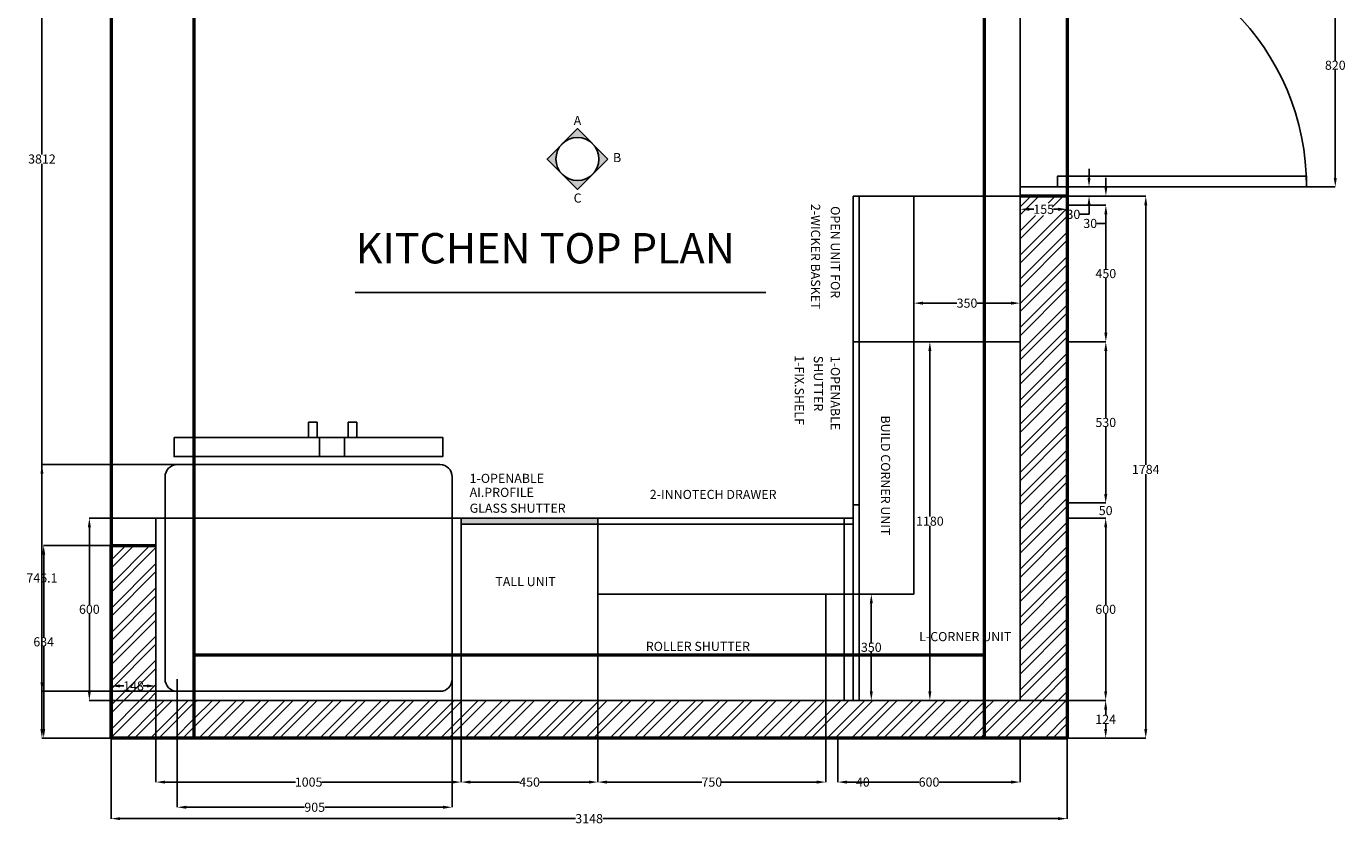
# Model space of a CAD drawing. Units: millimetres. Extents: x 26138 to 44889, y 15820 to 21179.
# Tile 1 of 8: x 26138 to 30481, y 15925 to 18552. Entities that reach past the tile are written whole.
import ezdxf

# ---------------------------------------------------------------- set-up
doc = ezdxf.new("R2010")
doc.units = ezdxf.units.MM
doc.header["$MEASUREMENT"] = 0
doc.header["$PDMODE"] = 3
for name, color, linetype, lineweight in [('A-ANNO-DIMS', 70, 'Continuous', 18), ('A-ANNO-TEXT', 7, 'Continuous', 18), ('A-DOOR', 4, 'Continuous', 25), ('A-FURN', 26, 'Continuous', 25), ('A-FURN-PATT', 40, 'Continuous', 13), ('A-WALL', 1, 'Continuous', 50), ('A-WALL-PATT', 8, 'Continuous', 13)]:
    doc.layers.add(name, color=color, linetype=linetype, lineweight=lineweight)
doc.styles.get("Standard").update_dxf_attribs({"font": 'arial.ttf'})
doc.dimstyles.get("Standard").update_dxf_attribs({"dimtxt": 30, "dimasz": 30, "dimexe": 0.18, "dimexo": 0.0625, "dimgap": 0.09, "dimtad": 0, "dimtih": 1, "dimtoh": 1, "dimdec": 0, "dimzin": 0, "dimdsep": 46, "dimtxsty": 'Standard', "dimcen": 0.09, "dimadec": 0, "dimazin": 0, "dimtfac": 1, "dimtdec": 0, "dimtofl": 0, "dimtmove": 0, "dimatfit": 3, "dimfxl": 1, "dimtolj": 1, "dimtzin": 0, "dimarcsym": 0})
pattern_1 = [(45, (-272.624, -1462.17), (-39.77476, 39.77476), []), (45, (-246.11, -1462.17), (-39.77476, 39.77476), [])]

# ---------------------------------------------------------------- blocks, each defined once
blk = doc.blocks.new('*U4')
for p, q in [((0, 0), (0, -6)), ((40, 0), (40, -6))]:
    blk.add_line(p, q)
blk.add_lwpolyline([(0, 0), (0, 40), (1.75, 40), (1.75, 0)], close=True)
blk.add_arc((0, 0), 40, 0, 90)
blk = doc.blocks.new('*D18')
at = {"layer": 'A-ANNO-DIMS', "color": 0, "lineweight": -2, "transparency": 16777216}
for p, q in [((29636.2, 18053.2), (29636.2, 18083.2)), ((29564.5, 18023.2), (29636.4, 18023.2)), ((29564.5, 17993.2), (29636.4, 17993.2)), ((29636.2, 17963.2), (29636.2, 17933.2)), ((29636.2, 17933.2), (29606.2, 17933.2))]:
    blk.add_line(p, q, dxfattribs=at)
at = {"layer": 'A-ANNO-DIMS', "color": 0, "transparency": 16777216}
for points in [[(29631.2, 18053.2), (29641.2, 18053.2), (29636.2, 18023.2)], [(29631.2, 17963.2), (29641.2, 17963.2), (29636.2, 17993.2)]]:
    blk.add_solid(points, dxfattribs=at)
at = {"layer": 'Defpoints', "color": 0, "transparency": 16777216}
for p in [(29564.5, 18023.2), (29564.5, 17993.2), (29636.2, 17993.2)]:
    blk.add_point(p, dxfattribs=at)
at = {"layer": 'A-ANNO-DIMS', "color": 0, "transparency": 16777216, "insert": (29584.7, 17933.2), "char_height": 30, "attachment_point": 5}
blk.add_mtext('\\A1;30', dxfattribs=at)
blk = doc.blocks.new('*D19')
at = {"layer": 'A-ANNO-DIMS', "color": 0, "lineweight": -2, "transparency": 16777216}
for p, q in [((29819.6, 18843.2), (30447, 18843.2)), ((30446.9, 18813.2), (30446.9, 18439.3)), ((30446.9, 18053.2), (30446.9, 18408.5)), ((30158.1, 18023.2), (30447, 18023.2))]:
    blk.add_line(p, q, dxfattribs=at)
at = {"layer": 'A-ANNO-DIMS', "color": 0, "transparency": 16777216}
for points in [[(30441.9, 18813.2), (30451.9, 18813.2), (30446.9, 18843.2)], [(30441.9, 18053.2), (30451.9, 18053.2), (30446.9, 18023.2)]]:
    blk.add_solid(points, dxfattribs=at)
at = {"layer": 'Defpoints', "color": 0, "transparency": 16777216}
for p in [(29819.5, 18843.2), (30158.1, 18023.2), (30446.9, 18023.2)]:
    blk.add_point(p, dxfattribs=at)
at = {"layer": 'A-ANNO-DIMS', "color": 0, "transparency": 16777216, "insert": (30446.9, 18423.9), "char_height": 30, "attachment_point": 5}
blk.add_mtext('\\A1;820', dxfattribs=at)
blk = doc.blocks.new('*D20')
at = {"layer": 'A-ANNO-DIMS', "color": 0, "lineweight": -2, "transparency": 16777216}
for p, q in [((29409.5, 17993.1), (29409.5, 17949.6)), ((29564.5, 17993.1), (29564.5, 17949.6)), ((29439.5, 17949.8), (29455, 17949.8)), ((29534.5, 17949.8), (29518.9, 17949.8))]:
    blk.add_line(p, q, dxfattribs=at)
at = {"layer": 'A-ANNO-DIMS', "color": 0, "transparency": 16777216}
for points in [[(29439.5, 17954.8), (29439.5, 17944.8), (29409.5, 17949.8)], [(29534.5, 17954.8), (29534.5, 17944.8), (29564.5, 17949.8)]]:
    blk.add_solid(points, dxfattribs=at)
at = {"layer": 'Defpoints', "color": 0, "transparency": 16777216}
for p in [(29409.5, 17993.2), (29564.5, 17993.2), (29564.5, 17949.8)]:
    blk.add_point(p, dxfattribs=at)
at = {"layer": 'A-ANNO-DIMS', "color": 0, "transparency": 16777216, "insert": (29487, 17949.8), "char_height": 30, "attachment_point": 5}
blk.add_mtext('\\A1;155', dxfattribs=at)
blk = doc.blocks.new('*D21')
at = {"layer": 'A-ANNO-DIMS', "color": 0, "lineweight": -2, "transparency": 16777216}
for p, q in [((29564.5, 17993.2), (29823.1, 17993.2)), ((29822.9, 17963.2), (29822.9, 17109)), ((29822.9, 16239.2), (29822.9, 17078.2)), ((29564.5, 16209.2), (29823.1, 16209.2))]:
    blk.add_line(p, q, dxfattribs=at)
at = {"layer": 'A-ANNO-DIMS', "color": 0, "transparency": 16777216}
for points in [[(29817.9, 17963.2), (29827.9, 17963.2), (29822.9, 17993.2)], [(29817.9, 16239.2), (29827.9, 16239.2), (29822.9, 16209.2)]]:
    blk.add_solid(points, dxfattribs=at)
at = {"layer": 'Defpoints', "color": 0, "transparency": 16777216}
for p in [(29564.5, 17993.2), (29564.5, 16209.2), (29822.9, 16209.2)]:
    blk.add_point(p, dxfattribs=at)
at = {"layer": 'A-ANNO-DIMS', "color": 0, "transparency": 16777216, "insert": (29822.9, 17093.6), "char_height": 30, "attachment_point": 5}
blk.add_mtext('\\A1;1784', dxfattribs=at)
blk = doc.blocks.new('*D22')
at = {"layer": 'A-ANNO-DIMS', "color": 0, "lineweight": -2, "transparency": 16777216}
for p, q in [((26416.4, 16843.2), (26194.7, 16843.2)), ((26194.9, 16813.2), (26194.9, 16541.6)), ((26194.9, 16239.2), (26194.9, 16510.8)), ((26416.4, 16209.2), (26194.7, 16209.2))]:
    blk.add_line(p, q, dxfattribs=at)
at = {"layer": 'A-ANNO-DIMS', "color": 0, "transparency": 16777216}
for points in [[(26189.9, 16813.2), (26199.9, 16813.2), (26194.9, 16843.2)], [(26189.9, 16239.2), (26199.9, 16239.2), (26194.9, 16209.2)]]:
    blk.add_solid(points, dxfattribs=at)
at = {"layer": 'Defpoints', "color": 0, "transparency": 16777216}
for p in [(26194.9, 16843.2), (26416.5, 16843.2), (26416.5, 16209.2)]:
    blk.add_point(p, dxfattribs=at)
at = {"layer": 'A-ANNO-DIMS', "color": 0, "transparency": 16777216, "insert": (26194.9, 16526.2), "char_height": 30, "attachment_point": 5}
blk.add_mtext('\\A1;634', dxfattribs=at)
blk = doc.blocks.new('*D23')
at = {"layer": 'A-ANNO-DIMS', "color": 0, "lineweight": -2, "transparency": 16777216}
for p, q in [((26564.4, 16933.2), (26345, 16933.2)), ((26345.1, 16903.2), (26345.1, 16648.6)), ((26345.1, 16363.2), (26345.1, 16617.8)), ((26564.4, 16333.2), (26345, 16333.2))]:
    blk.add_line(p, q, dxfattribs=at)
at = {"layer": 'A-ANNO-DIMS', "color": 0, "transparency": 16777216}
for points in [[(26340.1, 16903.2), (26350.1, 16903.2), (26345.1, 16933.2)], [(26340.1, 16363.2), (26350.1, 16363.2), (26345.1, 16333.2)]]:
    blk.add_solid(points, dxfattribs=at)
at = {"layer": 'Defpoints', "color": 0, "transparency": 16777216}
for p in [(26345.1, 16933.2), (26564.5, 16933.2), (26564.5, 16333.2)]:
    blk.add_point(p, dxfattribs=at)
at = {"layer": 'A-ANNO-DIMS', "color": 0, "transparency": 16777216, "insert": (26345.1, 16633.2), "char_height": 30, "attachment_point": 5}
blk.add_mtext('\\A1;600', dxfattribs=at)
blk = doc.blocks.new('*D24')
at = {"layer": 'A-ANNO-DIMS', "color": 0, "lineweight": -2, "transparency": 16777216}
for p, q in [((29564.5, 16333.2), (29691.2, 16333.2)), ((29691, 16303.2), (29691, 16286.4)), ((29691, 16239.2), (29691, 16256.1)), ((29564.5, 16209.2), (29691.2, 16209.2))]:
    blk.add_line(p, q, dxfattribs=at)
at = {"layer": 'A-ANNO-DIMS', "color": 0, "transparency": 16777216}
for points in [[(29686, 16303.2), (29696, 16303.2), (29691, 16333.2)], [(29686, 16239.2), (29696, 16239.2), (29691, 16209.2)]]:
    blk.add_solid(points, dxfattribs=at)
at = {"layer": 'Defpoints', "color": 0, "transparency": 16777216}
for p in [(29564.5, 16333.2), (29691, 16333.2), (29564.5, 16209.2)]:
    blk.add_point(p, dxfattribs=at)
at = {"layer": 'A-ANNO-DIMS', "color": 0, "transparency": 16777216, "insert": (29691, 16271.2), "char_height": 30, "attachment_point": 5}
blk.add_mtext('\\A1;124', dxfattribs=at)
blk = doc.blocks.new('*D25')
at = {"layer": 'A-ANNO-DIMS', "color": 0, "lineweight": -2, "transparency": 16777216}
for p, q in [((29564.5, 16933.2), (29691.2, 16933.2)), ((29691, 16903.2), (29691, 16648.6)), ((29691, 16363.2), (29691, 16617.8)), ((29564.5, 16333.2), (29691.2, 16333.2))]:
    blk.add_line(p, q, dxfattribs=at)
at = {"layer": 'A-ANNO-DIMS', "color": 0, "transparency": 16777216}
for points in [[(29686, 16903.2), (29696, 16903.2), (29691, 16933.2)], [(29686, 16363.2), (29696, 16363.2), (29691, 16333.2)]]:
    blk.add_solid(points, dxfattribs=at)
at = {"layer": 'Defpoints', "color": 0, "transparency": 16777216}
for p in [(29564.5, 16933.2), (29691, 16933.2), (29564.5, 16333.2)]:
    blk.add_point(p, dxfattribs=at)
at = {"layer": 'A-ANNO-DIMS', "color": 0, "transparency": 16777216, "insert": (29691, 16633.2), "char_height": 30, "attachment_point": 5}
blk.add_mtext('\\A1;600', dxfattribs=at)
blk = doc.blocks.new('*D26')
at = {"layer": 'A-ANNO-DIMS', "color": 0, "lineweight": -2, "transparency": 16777216}
for p, q in [((29691, 17013.2), (29691, 17043.2)), ((29564.5, 16983.2), (29691.2, 16983.2)), ((29564.5, 16933.2), (29691.2, 16933.2)), ((29691, 16903.2), (29691, 16873.2))]:
    blk.add_line(p, q, dxfattribs=at)
at = {"layer": 'A-ANNO-DIMS', "color": 0, "transparency": 16777216}
for points in [[(29686, 17013.2), (29696, 17013.2), (29691, 16983.2)], [(29686, 16903.2), (29696, 16903.2), (29691, 16933.2)]]:
    blk.add_solid(points, dxfattribs=at)
at = {"layer": 'Defpoints', "color": 0, "transparency": 16777216}
for p in [(29564.5, 16983.2), (29691, 16983.2), (29564.5, 16933.2)]:
    blk.add_point(p, dxfattribs=at)
at = {"layer": 'A-ANNO-DIMS', "color": 0, "transparency": 16777216, "insert": (29691, 16958.2), "char_height": 30, "attachment_point": 5}
blk.add_mtext('\\A1;50', dxfattribs=at)
blk = doc.blocks.new('*D27')
at = {"layer": 'A-ANNO-DIMS', "color": 0, "lineweight": -2, "transparency": 16777216}
for p, q in [((29564.5, 17513.2), (29691.6, 17513.2)), ((29691.4, 17483.2), (29691.4, 17263.6)), ((29691.4, 17013.2), (29691.4, 17232.8)), ((29564.5, 16983.2), (29691.6, 16983.2))]:
    blk.add_line(p, q, dxfattribs=at)
at = {"layer": 'A-ANNO-DIMS', "color": 0, "transparency": 16777216}
for points in [[(29686.4, 17483.2), (29696.4, 17483.2), (29691.4, 17513.2)], [(29686.4, 17013.2), (29696.4, 17013.2), (29691.4, 16983.2)]]:
    blk.add_solid(points, dxfattribs=at)
at = {"layer": 'Defpoints', "color": 0, "transparency": 16777216}
for p in [(29564.5, 17513.2), (29691.4, 17513.2), (29564.5, 16983.2)]:
    blk.add_point(p, dxfattribs=at)
at = {"layer": 'A-ANNO-DIMS', "color": 0, "transparency": 16777216, "insert": (29691.4, 17248.2), "char_height": 30, "attachment_point": 5}
blk.add_mtext('\\A1;530', dxfattribs=at)
blk = doc.blocks.new('*D28')
at = {"layer": 'A-ANNO-DIMS', "color": 0, "lineweight": -2, "transparency": 16777216}
for p, q in [((29564.5, 17963.2), (29691.7, 17963.2)), ((29691.6, 17933.2), (29691.6, 17753.6)), ((29691.6, 17543.2), (29691.6, 17722.8)), ((29564.5, 17513.2), (29691.7, 17513.2))]:
    blk.add_line(p, q, dxfattribs=at)
at = {"layer": 'A-ANNO-DIMS', "color": 0, "transparency": 16777216}
for points in [[(29686.6, 17933.2), (29696.6, 17933.2), (29691.6, 17963.2)], [(29686.6, 17543.2), (29696.6, 17543.2), (29691.6, 17513.2)]]:
    blk.add_solid(points, dxfattribs=at)
at = {"layer": 'Defpoints', "color": 0, "transparency": 16777216}
for p in [(29564.5, 17963.2), (29691.6, 17963.2), (29564.5, 17513.2)]:
    blk.add_point(p, dxfattribs=at)
at = {"layer": 'A-ANNO-DIMS', "color": 0, "transparency": 16777216, "insert": (29691.6, 17738.2), "char_height": 30, "attachment_point": 5}
blk.add_mtext('\\A1;450', dxfattribs=at)
blk = doc.blocks.new('*D29')
at = {"layer": 'A-ANNO-DIMS', "color": 0, "lineweight": -2, "transparency": 16777216}
for p, q in [((29691.7, 18023.2), (29691.7, 18053.2)), ((29564.5, 17993.2), (29691.9, 17993.2)), ((29564.5, 17963.2), (29691.9, 17963.2)), ((29691.7, 17903.2), (29661.7, 17903.2)), ((29691.7, 17933.2), (29691.7, 17903.2))]:
    blk.add_line(p, q, dxfattribs=at)
at = {"layer": 'A-ANNO-DIMS', "color": 0, "transparency": 16777216}
for points in [[(29686.7, 18023.2), (29696.7, 18023.2), (29691.7, 17993.2)], [(29686.7, 17933.2), (29696.7, 17933.2), (29691.7, 17963.2)]]:
    blk.add_solid(points, dxfattribs=at)
at = {"layer": 'Defpoints', "color": 0, "transparency": 16777216}
for p in [(29564.5, 17993.2), (29564.5, 17963.2), (29691.7, 17963.2)]:
    blk.add_point(p, dxfattribs=at)
at = {"layer": 'A-ANNO-DIMS', "color": 0, "transparency": 16777216, "insert": (29640.2, 17903.2), "char_height": 30, "attachment_point": 5}
blk.add_mtext('\\A1;30', dxfattribs=at)
blk = doc.blocks.new('*D30')
at = {"layer": 'A-ANNO-DIMS', "color": 0, "lineweight": -2, "transparency": 16777216}
for p, q in [((26416.5, 16333.3), (26416.5, 16381.1)), ((26446.5, 16380.9), (26458.6, 16380.9)), ((26534.5, 16380.9), (26522.3, 16380.9)), ((26564.5, 16333.3), (26564.5, 16381.1))]:
    blk.add_line(p, q, dxfattribs=at)
at = {"layer": 'A-ANNO-DIMS', "color": 0, "transparency": 16777216}
for points in [[(26446.5, 16385.9), (26446.5, 16375.9), (26416.5, 16380.9)], [(26534.5, 16385.9), (26534.5, 16375.9), (26564.5, 16380.9)]]:
    blk.add_solid(points, dxfattribs=at)
at = {"layer": 'Defpoints', "color": 0, "transparency": 16777216}
for p in [(26564.5, 16380.9), (26416.5, 16333.2), (26564.5, 16333.2)]:
    blk.add_point(p, dxfattribs=at)
at = {"layer": 'A-ANNO-DIMS', "color": 0, "transparency": 16777216, "insert": (26490.5, 16380.9), "char_height": 30, "attachment_point": 5}
blk.add_mtext('\\A1;148', dxfattribs=at)
blk = doc.blocks.new('*D31')
at = {"layer": 'A-ANNO-DIMS', "color": 0, "lineweight": -2, "transparency": 16777216}
for p, q in [((26564.5, 16209.1), (26564.5, 16064.3)), ((27569.5, 16209.1), (27569.5, 16064.3)), ((26594.5, 16064.5), (27023.4, 16064.5)), ((27539.5, 16064.5), (27110.5, 16064.5))]:
    blk.add_line(p, q, dxfattribs=at)
at = {"layer": 'A-ANNO-DIMS', "color": 0, "transparency": 16777216}
for points in [[(26594.5, 16069.5), (26594.5, 16059.5), (26564.5, 16064.5)], [(27539.5, 16069.5), (27539.5, 16059.5), (27569.5, 16064.5)]]:
    blk.add_solid(points, dxfattribs=at)
at = {"layer": 'Defpoints', "color": 0, "transparency": 16777216}
for p in [(26564.5, 16209.2), (27569.5, 16209.2), (27569.5, 16064.5)]:
    blk.add_point(p, dxfattribs=at)
at = {"layer": 'A-ANNO-DIMS', "color": 0, "transparency": 16777216, "insert": (27067, 16064.5), "char_height": 30, "attachment_point": 5}
blk.add_mtext('\\A1;1005', dxfattribs=at)
blk = doc.blocks.new('*D32')
at = {"layer": 'A-ANNO-DIMS', "color": 0, "lineweight": -2, "transparency": 16777216}
for p, q in [((27569.5, 16209.1), (27569.5, 16064.3)), ((28019.5, 16209.1), (28019.5, 16064.3)), ((27599.5, 16064.5), (27760.7, 16064.5)), ((27989.5, 16064.5), (27828.2, 16064.5))]:
    blk.add_line(p, q, dxfattribs=at)
at = {"layer": 'A-ANNO-DIMS', "color": 0, "transparency": 16777216}
for points in [[(27599.5, 16069.5), (27599.5, 16059.5), (27569.5, 16064.5)], [(27989.5, 16069.5), (27989.5, 16059.5), (28019.5, 16064.5)]]:
    blk.add_solid(points, dxfattribs=at)
at = {"layer": 'Defpoints', "color": 0, "transparency": 16777216}
for p in [(27569.5, 16209.2), (28019.5, 16209.2), (28019.5, 16064.5)]:
    blk.add_point(p, dxfattribs=at)
at = {"layer": 'A-ANNO-DIMS', "color": 0, "transparency": 16777216, "insert": (27794.5, 16064.5), "char_height": 30, "attachment_point": 5}
blk.add_mtext('\\A1;450', dxfattribs=at)
blk = doc.blocks.new('*D33')
at = {"layer": 'A-ANNO-DIMS', "color": 0, "lineweight": -2, "transparency": 16777216}
for p, q in [((28019.5, 16209.1), (28019.5, 16064.3)), ((28769.5, 16209.1), (28769.5, 16064.3)), ((28049.5, 16064.5), (28361.4, 16064.5)), ((28739.5, 16064.5), (28427.5, 16064.5))]:
    blk.add_line(p, q, dxfattribs=at)
at = {"layer": 'A-ANNO-DIMS', "color": 0, "transparency": 16777216}
for points in [[(28049.5, 16069.5), (28049.5, 16059.5), (28019.5, 16064.5)], [(28739.5, 16069.5), (28739.5, 16059.5), (28769.5, 16064.5)]]:
    blk.add_solid(points, dxfattribs=at)
at = {"layer": 'Defpoints', "color": 0, "transparency": 16777216}
for p in [(28019.5, 16209.2), (28769.5, 16209.2), (28769.5, 16064.5)]:
    blk.add_point(p, dxfattribs=at)
at = {"layer": 'A-ANNO-DIMS', "color": 0, "transparency": 16777216, "insert": (28394.5, 16064.5), "char_height": 30, "attachment_point": 5}
blk.add_mtext('\\A1;750', dxfattribs=at)
blk = doc.blocks.new('*D34')
at = {"layer": 'A-ANNO-DIMS', "color": 0, "lineweight": -2, "transparency": 16777216}
for p, q in [((28769.5, 16209.1), (28769.5, 16064.3)), ((28809.5, 16209.1), (28809.5, 16064.3)), ((28739.5, 16064.5), (28709.5, 16064.5)), ((28839.5, 16064.5), (28869.5, 16064.5))]:
    blk.add_line(p, q, dxfattribs=at)
at = {"layer": 'A-ANNO-DIMS', "color": 0, "transparency": 16777216}
for points in [[(28739.5, 16069.5), (28739.5, 16059.5), (28769.5, 16064.5)], [(28839.5, 16069.5), (28839.5, 16059.5), (28809.5, 16064.5)]]:
    blk.add_solid(points, dxfattribs=at)
at = {"layer": 'Defpoints', "color": 0, "transparency": 16777216}
for p in [(28769.5, 16209.2), (28809.5, 16209.2), (28809.5, 16064.5)]:
    blk.add_point(p, dxfattribs=at)
at = {"layer": 'A-ANNO-DIMS', "color": 0, "transparency": 16777216, "insert": (28891.6, 16064.5), "char_height": 30, "attachment_point": 5}
blk.add_mtext('\\A1;40', dxfattribs=at)
blk = doc.blocks.new('*D35')
at = {"layer": 'A-ANNO-DIMS', "color": 0, "lineweight": -2, "transparency": 16777216}
for p, q in [((28809.5, 16209.1), (28809.5, 16064.3)), ((29409.5, 16209.1), (29409.5, 16064.3)), ((28839.5, 16064.5), (29076.2, 16064.5)), ((29379.5, 16064.5), (29142.7, 16064.5))]:
    blk.add_line(p, q, dxfattribs=at)
at = {"layer": 'A-ANNO-DIMS', "color": 0, "transparency": 16777216}
for points in [[(28839.5, 16069.5), (28839.5, 16059.5), (28809.5, 16064.5)], [(29379.5, 16069.5), (29379.5, 16059.5), (29409.5, 16064.5)]]:
    blk.add_solid(points, dxfattribs=at)
at = {"layer": 'Defpoints', "color": 0, "transparency": 16777216}
for p in [(28809.5, 16209.2), (29409.5, 16209.2), (29409.5, 16064.5)]:
    blk.add_point(p, dxfattribs=at)
at = {"layer": 'A-ANNO-DIMS', "color": 0, "transparency": 16777216, "insert": (29109.5, 16064.5), "char_height": 30, "attachment_point": 5}
blk.add_mtext('\\A1;600', dxfattribs=at)
blk = doc.blocks.new('*D36')
at = {"layer": 'A-ANNO-DIMS', "color": 0, "lineweight": -2, "transparency": 16777216}
for p, q in [((26416.5, 16209.1), (26416.5, 15944.1)), ((29564.5, 16209.1), (29564.5, 15944.1)), ((26446.5, 15944.2), (27945.6, 15944.2)), ((29534.5, 15944.2), (28035.4, 15944.2))]:
    blk.add_line(p, q, dxfattribs=at)
at = {"layer": 'A-ANNO-DIMS', "color": 0, "transparency": 16777216}
for points in [[(26446.5, 15949.2), (26446.5, 15939.2), (26416.5, 15944.2)], [(29534.5, 15949.2), (29534.5, 15939.2), (29564.5, 15944.2)]]:
    blk.add_solid(points, dxfattribs=at)
at = {"layer": 'Defpoints', "color": 0, "transparency": 16777216}
for p in [(26416.5, 16209.2), (29564.5, 16209.2), (29564.5, 15944.2)]:
    blk.add_point(p, dxfattribs=at)
at = {"layer": 'A-ANNO-DIMS', "color": 0, "transparency": 16777216, "insert": (27990.5, 15944.2), "char_height": 30, "attachment_point": 5}
blk.add_mtext('\\A1;3148', dxfattribs=at)
blk = doc.blocks.new('*D37')
at = {"layer": 'A-ANNO-DIMS', "color": 0, "lineweight": -2, "transparency": 16777216}
for p, q in [((28919.5, 16683.2), (28919.6, 16683.2)), ((28919.4, 16653.2), (28919.4, 16523.6)), ((28919.4, 16363.2), (28919.4, 16492.8)), ((28919.5, 16333.2), (28919.6, 16333.2))]:
    blk.add_line(p, q, dxfattribs=at)
at = {"layer": 'A-ANNO-DIMS', "color": 0, "transparency": 16777216}
for points in [[(28914.4, 16653.2), (28924.4, 16653.2), (28919.4, 16683.2)], [(28914.4, 16363.2), (28924.4, 16363.2), (28919.4, 16333.2)]]:
    blk.add_solid(points, dxfattribs=at)
at = {"layer": 'Defpoints', "color": 0, "transparency": 16777216}
for p in [(28919.4, 16683.2), (28919.4, 16683.2), (28919.4, 16333.2)]:
    blk.add_point(p, dxfattribs=at)
at = {"layer": 'A-ANNO-DIMS', "color": 0, "transparency": 16777216, "insert": (28919.4, 16508.2), "char_height": 30, "attachment_point": 5}
blk.add_mtext('\\A1;350', dxfattribs=at)
blk = doc.blocks.new('*D38')
at = {"layer": 'A-ANNO-DIMS', "color": 0, "lineweight": -2, "transparency": 16777216}
for p, q in [((29059.5, 17513.1), (29059.5, 17641)), ((29089.5, 17640.8), (29201.3, 17640.8)), ((29379.5, 17640.8), (29267.6, 17640.8)), ((29409.5, 17513.3), (29409.5, 17641))]:
    blk.add_line(p, q, dxfattribs=at)
at = {"layer": 'A-ANNO-DIMS', "color": 0, "transparency": 16777216}
for points in [[(29089.5, 17645.8), (29089.5, 17635.8), (29059.5, 17640.8)], [(29379.5, 17645.8), (29379.5, 17635.8), (29409.5, 17640.8)]]:
    blk.add_solid(points, dxfattribs=at)
at = {"layer": 'Defpoints', "color": 0, "transparency": 16777216}
for p in [(29409.5, 17640.8), (29059.5, 17513), (29409.5, 17513.2)]:
    blk.add_point(p, dxfattribs=at)
at = {"layer": 'A-ANNO-DIMS', "color": 0, "transparency": 16777216, "insert": (29234.5, 17640.8), "char_height": 30, "attachment_point": 5}
blk.add_mtext('\\A1;350', dxfattribs=at)
blk = doc.blocks.new('*D39')
at = {"layer": 'A-ANNO-DIMS', "color": 0, "lineweight": -2, "transparency": 16777216}
for p, q in [((29406.3, 17513.2), (29112, 17513.2)), ((29112.2, 17483.2), (29112.2, 16938.6)), ((29112.2, 16363.2), (29112.2, 16907.8)), ((29406.3, 16333.2), (29112, 16333.2))]:
    blk.add_line(p, q, dxfattribs=at)
at = {"layer": 'A-ANNO-DIMS', "color": 0, "transparency": 16777216}
for points in [[(29107.2, 17483.2), (29117.2, 17483.2), (29112.2, 17513.2)], [(29107.2, 16363.2), (29117.2, 16363.2), (29112.2, 16333.2)]]:
    blk.add_solid(points, dxfattribs=at)
at = {"layer": 'Defpoints', "color": 0, "transparency": 16777216}
for p in [(29112.2, 17513.2), (29406.4, 17513.2), (29406.4, 16333.2)]:
    blk.add_point(p, dxfattribs=at)
at = {"layer": 'A-ANNO-DIMS', "color": 0, "transparency": 16777216, "insert": (29112.2, 16923.2), "char_height": 30, "attachment_point": 5}
blk.add_mtext('\\A1;1180', dxfattribs=at)
blk = doc.blocks.new('*D131')
at = {"layer": 'A-ANNO-DIMS', "color": 0, "lineweight": -2, "transparency": 16777216}
for p, q in [((26416.4, 20021.2), (26188.8, 20021.2)), ((26189, 19991.2), (26189, 18130.6)), ((26189, 16239.2), (26189, 18099.8)), ((26416.4, 16209.2), (26188.8, 16209.2))]:
    blk.add_line(p, q, dxfattribs=at)
at = {"layer": 'A-ANNO-DIMS', "color": 0, "transparency": 16777216}
for points in [[(26184, 19991.2), (26194, 19991.2), (26189, 20021.2)], [(26184, 16239.2), (26194, 16239.2), (26189, 16209.2)]]:
    blk.add_solid(points, dxfattribs=at)
at = {"layer": 'Defpoints', "color": 0, "transparency": 16777216}
for p in [(26416.5, 20021.2), (26189, 16209.2), (26416.5, 16209.2)]:
    blk.add_point(p, dxfattribs=at)
at = {"layer": 'A-ANNO-DIMS', "color": 0, "transparency": 16777216, "insert": (26189, 18115.2), "char_height": 30, "attachment_point": 5}
blk.add_mtext('\\A1;3812', dxfattribs=at)
blk = doc.blocks.new('*D132')
at = {"layer": 'A-ANNO-DIMS', "color": 0, "lineweight": -2, "transparency": 16777216}
for p, q in [((26634.5, 16403.1), (26634.5, 15981.5)), ((27539.5, 16403.1), (27539.5, 15981.5)), ((26664.5, 15981.7), (27053.6, 15981.7)), ((27509.5, 15981.7), (27120.3, 15981.7))]:
    blk.add_line(p, q, dxfattribs=at)
at = {"layer": 'A-ANNO-DIMS', "color": 0, "transparency": 16777216}
for points in [[(26664.5, 15986.7), (26664.5, 15976.7), (26634.5, 15981.7)], [(27509.5, 15986.7), (27509.5, 15976.7), (27539.5, 15981.7)]]:
    blk.add_solid(points, dxfattribs=at)
at = {"layer": 'Defpoints', "color": 0, "transparency": 16777216}
for p in [(26634.5, 16403.2), (27539.5, 16403.2), (27539.5, 15981.7)]:
    blk.add_point(p, dxfattribs=at)
at = {"layer": 'A-ANNO-DIMS', "color": 0, "transparency": 16777216, "insert": (27087, 15981.7), "char_height": 30, "attachment_point": 5}
blk.add_mtext('\\A1;905', dxfattribs=at)
blk = doc.blocks.new('*D133')
at = {"layer": 'A-ANNO-DIMS', "color": 0, "lineweight": -2, "transparency": 16777216}
for p, q in [((26634.4, 17109.3), (26188.8, 17109.3)), ((26189, 17079.3), (26189, 16751.7)), ((26189, 16393.2), (26189, 16720.9)), ((26634.4, 16363.2), (26188.8, 16363.2))]:
    blk.add_line(p, q, dxfattribs=at)
at = {"layer": 'A-ANNO-DIMS', "color": 0, "transparency": 16777216}
for points in [[(26184, 17079.3), (26194, 17079.3), (26189, 17109.3)], [(26184, 16393.2), (26194, 16393.2), (26189, 16363.2)]]:
    blk.add_solid(points, dxfattribs=at)
at = {"layer": 'Defpoints', "color": 0, "transparency": 16777216}
for p in [(26634.5, 17109.3), (26189, 16363.2), (26634.5, 16363.2)]:
    blk.add_point(p, dxfattribs=at)
at = {"layer": 'A-ANNO-DIMS', "color": 0, "transparency": 16777216, "insert": (26189, 16736.3), "char_height": 30, "attachment_point": 5}
blk.add_mtext('\\A1;746.1', dxfattribs=at)

msp = doc.modelspace()

# ---------------------------------------------------------------- hatches: boundary and pattern name
at = {"layer": 'A-FURN-PATT'}
h = msp.add_hatch(color=256, dxfattribs=at)
h.dxf.hatch_style = 1
h.paths.add_polyline_path([(27901.932, 18165.203, -0.41421356), (28001.932, 18165.203), (27951.932, 18215.203)])
h = msp.add_hatch(color=256, dxfattribs=at)
h.dxf.hatch_style = 1
h.paths.add_polyline_path([(27881.222, 18115.203, -0.19891237), (27901.932, 18165.203), (27851.932, 18115.203), (27901.932, 18065.203, -0.19891237)])
h = msp.add_hatch(color=256, dxfattribs=at)
h.dxf.hatch_style = 1
h.paths.add_polyline_path([(28001.932, 18165.203, -0.19891237), (28022.643, 18115.203, -0.19891237), (28001.932, 18065.203), (28051.932, 18115.203)])
h = msp.add_hatch(color=256, dxfattribs=at)
h.dxf.hatch_style = 1
h.paths.add_polyline_path([(28001.932, 18065.203, -0.41421356), (27901.932, 18065.203), (27951.932, 18015.203)])
h = msp.add_hatch(color=256, dxfattribs=at)
h.dxf.hatch_style = 1
h.paths.add_polyline_path([(27569.457, 16933.203), (27569.457, 16913.203), (28019.457, 16913.203), (28019.457, 16933.203)])
at = {"layer": 'A-WALL-PATT'}
h = msp.add_hatch(dxfattribs=at)
h.set_pattern_fill('ANSI32', color=256, scale=150)
h.set_pattern_definition(pattern_1)
h.paths.add_polyline_path([(29564.457, 17993.203), (29409.457, 17993.203), (29409.457, 16333.203), (29564.457, 16333.203)])
h.paths.add_polyline_path([(29457.687, 17929.054), (29514.304, 17929.054), (29514.304, 17970.268), (29457.687, 17970.268)], flags=16)
h = msp.add_hatch(dxfattribs=at)
h.set_pattern_fill('ANSI32', color=256, scale=150)
h.set_pattern_definition(pattern_1)
h.paths.add_polyline_path([(26416.457, 16333.203), (26564.457, 16333.203), (26564.457, 16843.203), (26416.457, 16843.203)])
h = msp.add_hatch(dxfattribs=at)
h.set_pattern_fill('ANSI32', color=256, scale=150)
h.set_pattern_definition(pattern_1)
h.paths.add_polyline_path([(26564.457, 16333.203), (26416.457, 16333.203), (26416.457, 16209.203), (26564.457, 16209.203)])
h = msp.add_hatch(dxfattribs=at)
h.set_pattern_fill('ANSI32', color=256, scale=150)
h.set_pattern_definition(pattern_1)
h.paths.add_polyline_path([(26689.457, 16333.203), (26564.457, 16333.203), (26564.457, 16209.203), (26689.457, 16209.203)])
h = msp.add_hatch(dxfattribs=at)
h.set_pattern_fill('ANSI32', color=256, scale=150)
h.set_pattern_definition(pattern_1)
h.paths.add_polyline_path([(29291.457, 16333.203), (26689.457, 16333.203), (26689.457, 16209.203), (29291.457, 16209.203)])
h = msp.add_hatch(dxfattribs=at)
h.set_pattern_fill('ANSI32', color=256, scale=150)
h.set_pattern_definition(pattern_1)
h.paths.add_polyline_path([(29564.457, 16333.203), (29291.457, 16333.203), (29291.457, 16209.203), (29564.457, 16209.203)])

# ---------------------------------------------------------------- linework, layer by layer
at = {"layer": 'A-FURN'}
for p, q in [((29409.457, 19792.203), (29409.457, 16333.203)), ((29409.457, 17993.203), (28859.667, 17993.203)), ((28859.667, 17993.203), (28859.667, 16333.203)), ((28879.667, 17993.203), (28879.667, 16333.203)), ((29059.457, 17993.203), (29059.487, 17513.025)), ((27220.069, 17675.648), (28572.332, 17675.648)), ((29059.667, 17640.783), (29059.667, 16683.203)), ((29406.396, 17513.203), (28859.667, 17513.203)), ((27066.411, 17199.124), (27066.411, 17249.124)), ((27066.411, 17199.124), (27066.411, 17249.124)), ((27066.411, 17249.124), (27094.964, 17249.124)), ((27094.964, 17249.124), (27094.964, 17199.124)), ((27197.118, 17199.124), (27197.118, 17249.124)), ((27197.118, 17199.124), (27197.118, 17249.124)), ((27197.118, 17249.124), (27225.671, 17249.124)), ((27225.671, 17249.124), (27225.671, 17199.124)), ((27102.526, 17199.124), (27102.526, 17136.055)), ((27184.859, 17199.124), (27184.859, 17136.055)), ((26594.457, 16403.203), (26594.457, 17069.33)), ((27499.457, 17109.33), (26634.457, 17109.33)), ((27539.457, 16403.203), (27539.457, 17069.33)), ((28859.667, 16977.268), (28879.667, 16977.268)), ((26564.457, 16843.203), (26564.457, 16933.203)), ((26564.457, 16933.203), (28859.667, 16933.203)), ((27569.457, 16209.203), (27569.457, 16933.203)), ((27569.457, 16933.203), (28019.457, 16933.203)), ((27569.457, 16913.203), (28859.667, 16913.203)), ((28019.457, 16933.203), (28019.457, 16209.203)), ((28829.667, 16913.203), (28829.667, 16933.203)), ((28859.667, 16913.203), (28829.667, 16913.203)), ((28829.667, 16913.203), (28829.667, 16333.203)), ((26564.457, 16843.203), (26564.457, 16209.203)), ((28019.457, 16683.203), (28769.457, 16683.203)), ((28769.457, 16209.203), (28769.457, 16683.203)), ((28769.457, 16683.203), (29059.667, 16683.203)), ((29564.457, 16333.203), (26416.457, 16333.203)), ((26634.457, 16363.203), (27499.457, 16363.203))]:
    msp.add_line(p, q, dxfattribs=at)
for points in [[(28051.932, 18115.203), (27951.932, 18215.203), (27851.932, 18115.203), (27951.932, 18015.203)], [(26624.086, 17199.124), (27508.736, 17199.124), (27508.736, 17136.055), (26624.086, 17136.055)]]:
    msp.add_lwpolyline(points, close=True, dxfattribs=at)
msp.add_circle((27951.932, 18115.203), 70.711, dxfattribs=at)
for centre, start, end in [((26634.457, 17069.33), 90, 180), ((27499.457, 17069.33), 0, 90), ((26634.457, 16403.203), 180, 270), ((27499.457, 16403.203), 270, 0)]:
    msp.add_arc(centre, 40, start, end, dxfattribs=at)
at = {"layer": 'A-WALL'}
for p, q in [((29291.457, 20021.203), (29291.457, 16209.203)), ((29564.457, 20021.203), (29564.457, 16209.203)), ((26689.457, 19442.203), (26689.457, 16209.203)), ((26416.457, 19352.203), (26416.457, 16209.203)), ((29564.457, 17993.203), (29409.457, 17993.203)), ((26416.457, 16209.203), (26416.457, 16843.203)), ((26416.457, 16843.203), (26564.457, 16843.203)), ((29291.457, 16482.203), (26689.457, 16482.203)), ((29564.457, 16209.203), (26416.457, 16209.203))]:
    msp.add_line(p, q, dxfattribs=at)

# ---------------------------------------------------------------- block references
at = {"layer": 'A-DOOR', "xscale": -20.5, "yscale": 20.5, "zscale": 20.5, "rotation": 270}
msp.add_blockref('*U4', (29532.457, 18023.203), dxfattribs=at)

# ---------------------------------------------------------------- texts
at = {"layer": 'A-ANNO-TEXT'}
for s, height, p in [('A', 30, (27939.695, 18227.075)), ('B ', 30, (28069.231, 18104.863)), ('C ', 30, (27939.365, 17971.833)), ('KITCHEN TOP PLAN', 100, (27222.141, 17771.475)), ('1-OPENABLE  ', 30, (27597.091, 17049.151)), ('AI.PROFILE', 30, (27597.091, 17003.049)), ('2-INNOTECH DRAWER', 30, (28190.185, 16996.216)), ('GLASS SHUTTER  ', 30, (27597.091, 16950.959)), ('TALL UNIT', 30, (27681.878, 16709.481)), ('L-CORNER UNIT', 30, (29076.937, 16528.305)), ('ROLLER SHUTTER', 30, (28177.029, 16496.234))]:
    msp.add_text(s, height=height, dxfattribs=at).set_placement(p)
for s, p in [('2-WICKER BASKET', (28720.985, 17967.628)), ('OPEN UNIT FOR ', (28786.049, 17959.987)), ('1-FIX.SHELF', (28667.594, 17469.261)), ('SHUTTER', (28730.247, 17467.569)), ('1-OPENABLE', (28786.049, 17467.569)), ('BUILD CORNER UNIT', (28951.398, 17271.25))]:
    msp.add_text(s, height=30, rotation=270, dxfattribs=at).set_placement(p)

# ---------------------------------------------------------------- dimensions: what is measured, and where the dimension line sits
at = {"layer": 'A-ANNO-DIMS'}
for base, p1, p2, override, picture, middle in [((26188.957, 16209.203), (26416.457, 20021.203), (26416.457, 16209.203), {"dimdec": 0, "dimlfac": 1, "dimrnd": 0, "dimzin": 0, "dimdsep": 46, "dimlunit": 2}, '*D131', (26188.957, 18115.203)), ((29636.25, 17993.203), (29564.457, 18023.203), (29564.457, 17993.203), {"dimclrd": 0, "dimclre": 0, "dimclrt": 0}, '*D18', (29584.734, 17933.203)), ((29691.741, 17963.203), (29564.457, 17993.203), (29564.457, 17963.203), {"dimclrd": 0, "dimclre": 0, "dimclrt": 0}, '*D29', (29640.225, 17903.203)), ((29691.561, 17963.203), (29564.457, 17513.203), (29564.457, 17963.203), {"dimclrd": 0, "dimclre": 0, "dimclrt": 0}, '*D28', (29691.561, 17738.203)), ((29691.381, 17513.203), (29564.457, 16983.203), (29564.457, 17513.203), {"dimclrd": 0, "dimclre": 0, "dimclrt": 0}, '*D27', (29691.381, 17248.203)), ((26188.957, 16363.203), (26634.457, 17109.33), (26634.457, 16363.203), {"dimdec": 1, "dimlfac": 1, "dimrnd": 0, "dimzin": 0, "dimdsep": 46, "dimlunit": 2}, '*D133', (26188.957, 16736.266)), ((29691.001, 16983.203), (29564.457, 16933.203), (29564.457, 16983.203), {"dimclrd": 0, "dimclre": 0, "dimclrt": 0}, '*D26', (29691.001, 16958.203)), ((29691.001, 16933.203), (29564.457, 16333.203), (29564.457, 16933.203), {"dimclrd": 0, "dimclre": 0, "dimclrt": 0}, '*D25', (29691.001, 16633.203)), ((28919.413, 16683.203), (28919.413, 16333.203), (28919.413, 16683.203), {"dimclrd": 0, "dimclre": 0, "dimclrt": 0}, '*D37', (28919.413, 16508.203)), ((29691.001, 16333.203), (29564.457, 16209.203), (29564.457, 16333.203), {"dimclrd": 0, "dimclre": 0, "dimclrt": 0}, '*D24', (29691.001, 16271.203))]:
    dim = msp.add_linear_dim(base=base, p1=p1, p2=p2, angle=90, dimstyle='Standard', override=override, dxfattribs=at)
    dim.commit()
    dim.dimension.update_dxf_attribs({"geometry": picture, "text_midpoint": middle})
for base, p1, p2, picture, middle in [((30446.851, 18023.203), (29819.535, 18843.203), (30158.053, 18023.203), '*D19', (30446.851, 18423.9)), ((29822.948, 16209.203), (29564.457, 17993.203), (29564.457, 16209.203), '*D21', (29822.948, 17093.619)), ((29112.226, 17513.203), (29406.396, 16333.203), (29406.396, 17513.203), '*D39', (29112.226, 16923.203)), ((26345.142, 16933.203), (26564.457, 16333.203), (26564.457, 16933.203), '*D23', (26345.142, 16633.203)), ((26194.915, 16843.203), (26416.457, 16209.203), (26416.457, 16843.203), '*D22', (26194.915, 16526.203))]:
    dim = msp.add_linear_dim(base=base, p1=p1, p2=p2, angle=90, dimstyle='Standard', override={"dimclrd": 0, "dimclre": 0, "dimclrt": 0}, dxfattribs=at)
    dim.commit()
    dim.dimension.update_dxf_attribs({"geometry": picture, "text_midpoint": middle, "dimtype": 160})
for base, p1, p2, override, picture, middle in [((29564.457, 17949.804), (29409.457, 17993.203), (29564.457, 17993.203), {"dimclrd": 0, "dimclre": 0, "dimclrt": 0}, '*D20', (29486.957, 17949.804)), ((29409.457, 17640.813), (29059.487, 17513.025), (29409.457, 17513.203), {"dimclrd": 0, "dimclre": 0, "dimclrt": 0}, '*D38', (29234.472, 17640.813)), ((26564.457, 16380.933), (26416.457, 16333.203), (26564.457, 16333.203), {"dimclrd": 0, "dimclre": 0, "dimclrt": 0}, '*D30', (26490.457, 16380.933)), ((27539.457, 15981.703), (26634.457, 16403.203), (27539.457, 16403.203), {"dimdec": 0, "dimlfac": 1, "dimrnd": 0, "dimzin": 0, "dimdsep": 46, "dimlunit": 2}, '*D132', (27086.957, 15981.703)), ((29564.457, 15944.235), (26416.457, 16209.203), (29564.457, 16209.203), {"dimclrd": 0, "dimclre": 0, "dimclrt": 0}, '*D36', (27990.457, 15944.235)), ((27569.457, 16064.479), (26564.457, 16209.203), (27569.457, 16209.203), {"dimclrd": 0, "dimclre": 0, "dimclrt": 0}, '*D31', (27066.957, 16064.479)), ((28019.457, 16064.509), (27569.457, 16209.203), (28019.457, 16209.203), {"dimclrd": 0, "dimclre": 0, "dimclrt": 0}, '*D32', (27794.457, 16064.509)), ((28769.457, 16064.509), (28019.457, 16209.203), (28769.457, 16209.203), {"dimclrd": 0, "dimclre": 0, "dimclrt": 0}, '*D33', (28394.457, 16064.509)), ((28809.457, 16064.479), (28769.457, 16209.203), (28809.457, 16209.203), {"dimclrd": 0, "dimclre": 0, "dimclrt": 0}, '*D34', (28891.587, 16064.479)), ((29409.457, 16064.479), (28809.457, 16209.203), (29409.457, 16209.203), {"dimclrd": 0, "dimclre": 0, "dimclrt": 0}, '*D35', (29109.457, 16064.479))]:
    dim = msp.add_linear_dim(base=base, p1=p1, p2=p2, dimstyle='Standard', override=override, dxfattribs=at)
    dim.commit()
    dim.dimension.update_dxf_attribs({"geometry": picture, "text_midpoint": middle})

doc.saveas('drawing.dxf')
